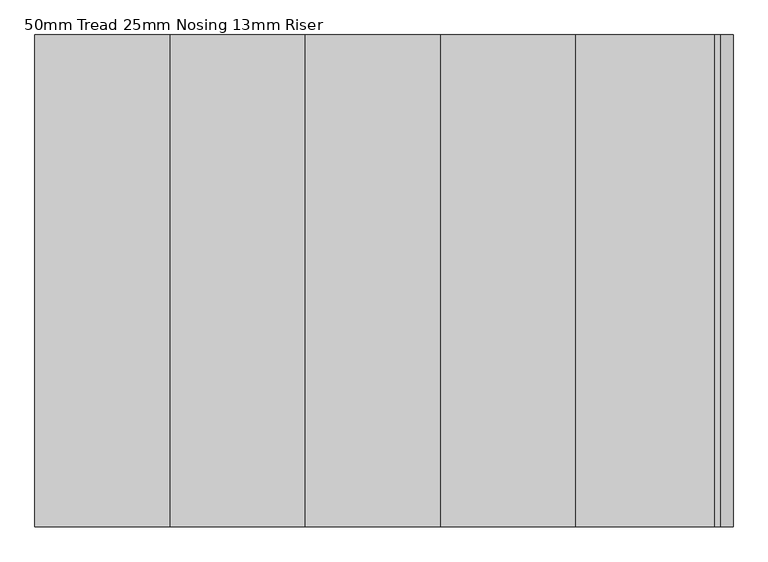
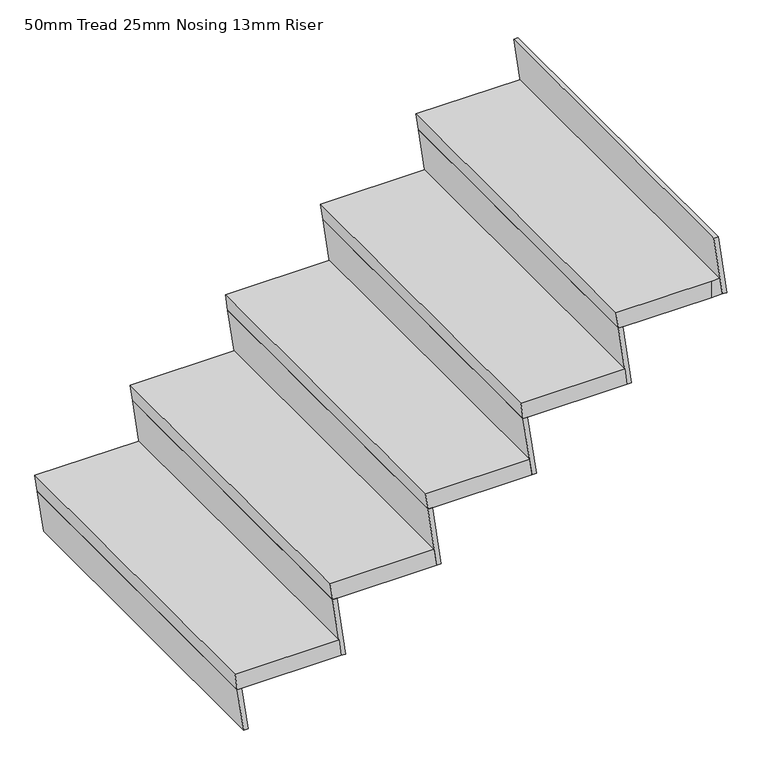
"""IFC4 building model written with IfcOpenShell, lengths in millimetres: stair flight geometry, 50mm Tread 25mm Nosing 13mm Riser."""

from ifc_helpers import new_model, si_unit, origin, place, context, project, spatial, faceted_brep, source, transform, mapped, element, save


def stair_flight_50mm_tread_25mm_nosing_13mm_riser_d89b79ae(model_context):
    return source(origin(), model_context, "Body", "Brep", [
        faceted_brep([(12125.7864069, -3533.7536983, 179.2941176), (12132.7581917, -3533.7536983, 129.2941176), (12132.7581917, -2533.727917, 129.2941176), (12125.7864069, -2533.727917, 179.2941176), (11825.7864069, -2533.727917, 179.2941176), (11825.7864069, -3533.7536983, 179.2941176), (11832.7581917, -3533.7536983, 129.2941176), (11832.7581917, -2533.727917, 129.2941176)], [[[0, 1, 2, 3]], [[3, 4, 5, 0]], [[2, 1, 6, 7]], [[4, 3, 2, 7]], [[0, 5, 6, 1]], [[5, 4, 7, 6]]]),
        faceted_brep([(11832.7581917, -3533.7536983, 129.2941176), (11850.7864069, -3533.7536983, 0.0), (11863.4073364, -3533.7536983, 0.0), (11845.3791212, -3533.7536983, 129.2941176), (11832.7581917, -2533.727917, 129.2941176), (11845.3791212, -2533.727917, 129.2941176), (11863.4073364, -2533.727917, 0.0), (11850.7864069, -2533.727917, 0.0)], [[[0, 1, 2, 3]], [[4, 5, 6, 7]], [[1, 0, 4, 7]], [[2, 1, 7, 6]], [[3, 2, 6, 5]], [[0, 3, 5, 4]]]),
        faceted_brep([(12107.7581917, -3533.7536983, 308.5882353), (12132.7581917, -3533.7536983, 129.2941176), (12145.3791212, -3533.7536983, 129.2941176), (12120.3791212, -3533.7536983, 308.5882353), (12107.7581917, -2533.727917, 308.5882353), (12120.3791212, -2533.727917, 308.5882353), (12145.3791212, -2533.727917, 129.2941176), (12132.7581917, -2533.727917, 129.2941176)], [[[0, 1, 2, 3]], [[4, 5, 6, 7]], [[1, 0, 4, 7]], [[2, 1, 7, 6]], [[3, 2, 6, 5]], [[0, 3, 5, 4]]]),
        faceted_brep([(12400.7864069, -2533.727917, 358.5882353), (12100.7864069, -2533.727917, 358.5882353), (12100.7864069, -3533.7536983, 358.5882353), (12400.7864069, -3533.7536983, 358.5882353), (12407.7581917, -2533.727917, 308.5882353), (12407.7581917, -3533.7536983, 308.5882353), (12107.7581917, -3533.7536983, 308.5882353), (12107.7581917, -2533.727917, 308.5882353)], [[[0, 1, 2, 3]], [[4, 5, 6, 7]], [[1, 0, 4, 7]], [[3, 2, 6, 5]], [[3, 5, 4, 0]], [[2, 1, 7, 6]]]),
        faceted_brep([(12382.7581917, -3533.7536983, 487.8823529), (12407.7581917, -3533.7536983, 308.5882353), (12420.3791212, -3533.7536983, 308.5882353), (12395.3791212, -3533.7536983, 487.8823529), (12382.7581917, -2533.727917, 487.8823529), (12395.3791212, -2533.727917, 487.8823529), (12420.3791212, -2533.727917, 308.5882353), (12407.7581917, -2533.727917, 308.5882353)], [[[0, 1, 2, 3]], [[4, 5, 6, 7]], [[1, 0, 4, 7]], [[2, 1, 7, 6]], [[3, 2, 6, 5]], [[0, 3, 5, 4]]]),
        faceted_brep([(12675.7864069, -2533.727917, 537.8823529), (12375.7864069, -2533.727917, 537.8823529), (12375.7864069, -3533.7536983, 537.8823529), (12675.7864069, -3533.7536983, 537.8823529), (12682.7581917, -2533.727917, 487.8823529), (12682.7581917, -3533.7536983, 487.8823529), (12382.7581917, -3533.7536983, 487.8823529), (12382.7581917, -2533.727917, 487.8823529)], [[[0, 1, 2, 3]], [[4, 5, 6, 7]], [[1, 0, 4, 7]], [[3, 2, 6, 5]], [[3, 5, 4, 0]], [[2, 1, 7, 6]]]),
        faceted_brep([(12657.7581917, -3533.7536983, 667.1764706), (12682.7581917, -3533.7536983, 487.8823529), (12695.3791212, -3533.7536983, 487.8823529), (12670.3791212, -3533.7536983, 667.1764706), (12657.7581917, -2533.727917, 667.1764706), (12670.3791212, -2533.727917, 667.1764706), (12695.3791212, -2533.727917, 487.8823529), (12682.7581917, -2533.727917, 487.8823529)], [[[0, 1, 2, 3]], [[4, 5, 6, 7]], [[1, 0, 4, 7]], [[2, 1, 7, 6]], [[3, 2, 6, 5]], [[0, 3, 5, 4]]]),
        faceted_brep([(12950.7864069, -2533.727917, 717.1764706), (12650.7864069, -2533.727917, 717.1764706), (12650.7864069, -3533.7536983, 717.1764706), (12950.7864069, -3533.7536983, 717.1764706), (12957.7581917, -2533.727917, 667.1764706), (12957.7581917, -3533.7536983, 667.1764706), (12657.7581917, -3533.7536983, 667.1764706), (12657.7581917, -2533.727917, 667.1764706)], [[[0, 1, 2, 3]], [[4, 5, 6, 7]], [[1, 0, 4, 7]], [[3, 2, 6, 5]], [[3, 5, 4, 0]], [[2, 1, 7, 6]]]),
        faceted_brep([(12932.7581917, -3533.7536983, 846.4705882), (12957.7581917, -3533.7536983, 667.1764706), (12970.3791212, -3533.7536983, 667.1764706), (12945.3791212, -3533.7536983, 846.4705882), (12932.7581917, -2533.727917, 846.4705882), (12945.3791212, -2533.727917, 846.4705882), (12970.3791212, -2533.727917, 667.1764706), (12957.7581917, -2533.727917, 667.1764706)], [[[0, 1, 2, 3]], [[4, 5, 6, 7]], [[1, 0, 4, 7]], [[2, 1, 7, 6]], [[3, 2, 6, 5]], [[0, 3, 5, 4]]]),
        faceted_brep([(13207.7581917, -3533.7536983, 1025.7647059), (13232.7581917, -3533.7536983, 846.4705882), (13245.3791212, -3533.7536983, 846.4705882), (13220.3791212, -3533.7536983, 1025.7647059), (13207.7581917, -2533.727917, 1025.7647059), (13220.3791212, -2533.727917, 1025.7647059), (13245.3791212, -2533.727917, 846.4705882), (13232.7581917, -2533.727917, 846.4705882)], [[[0, 1, 2, 3]], [[4, 5, 6, 7]], [[1, 0, 4, 7]], [[2, 1, 7, 6]], [[3, 2, 6, 5]], [[0, 3, 5, 4]]]),
        faceted_brep([(13225.7864069, -2533.727917, 896.4705882), (12925.7864069, -2533.727917, 896.4705882), (12925.7864069, -3533.7536983, 896.4705882), (13200.7864069, -3533.7536983, 896.4705882), (13225.7864069, -3533.7536983, 896.4705882), (13232.7581917, -2533.727917, 846.4705882), (13232.7581917, -3533.7536983, 846.4705882), (13200.7864069, -3533.7536983, 846.4705882), (12932.7581917, -3533.7536983, 846.4705882), (12932.7581917, -2533.727917, 846.4705882)], [[[0, 1, 2, 3, 4]], [[5, 6, 7, 8, 9]], [[1, 0, 5, 9]], [[3, 2, 8, 7]], [[4, 3, 7, 6]], [[4, 6, 5, 0]], [[2, 1, 9, 8]]]),
    ])


if __name__ == "__main__":
    model = new_model("IFC4")
    model_context = context("Model", 3, world=origin())
    ifc_project = project(units=[si_unit("LENGTHUNIT", "METRE", prefix="MILLI")], contexts=[model_context])
    site = spatial("IfcSite", under=ifc_project)
    building = spatial("IfcBuilding", under=site)
    placement = place(None, origin())
    stair_flight_50mm_tread_25mm_nosing_13mm_riser_shape = stair_flight_50mm_tread_25mm_nosing_13mm_riser_d89b79ae(model_context)
    element("IfcStairFlight", 1, ObjectType="50mm Tread 25mm Nosing 13mm Riser", at=placement, inside=building, context=model_context, shape_type="MappedRepresentation", body=[
        mapped(stair_flight_50mm_tread_25mm_nosing_13mm_riser_shape, transform((0.0, 0.0, 0.0), x_axis=(1.0, 0.0, 0.0), y_axis=(0.0, 1.0, 0.0), z_axis=(0.0, 0.0, 1.0))),
    ])
    save(model, "model.ifc")
